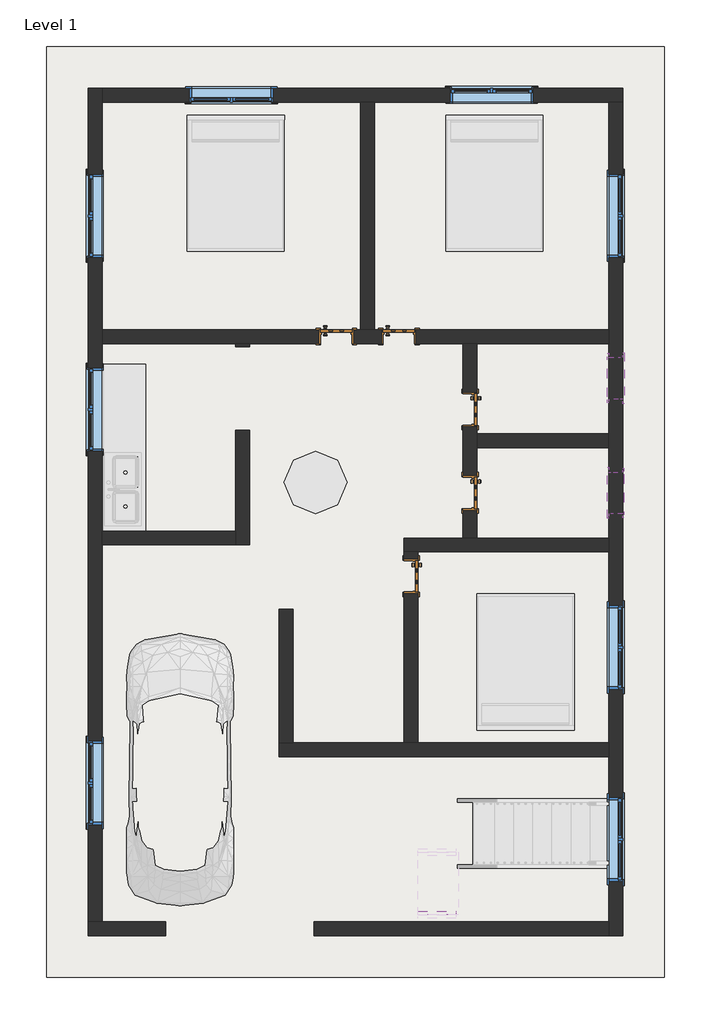
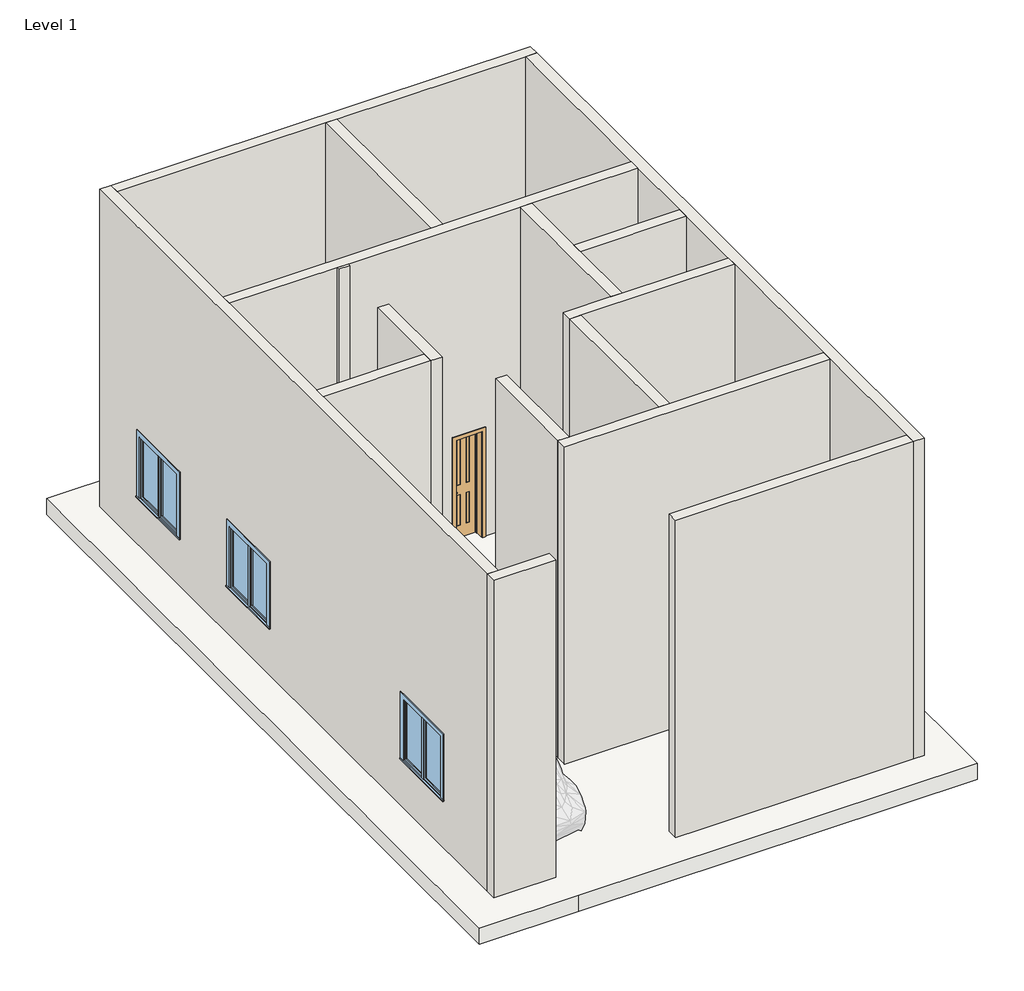
# One storey, part 1 of 2: 16 walls, 10 windows, 5 doors, 1 railing, 1 slab.
"""IFC4 building model written with IfcOpenShell, lengths in millimetres."""

from ifc_helpers import new_model, si_unit, frame, origin, origin_with_axes, place, context, project, spatial, polyline, outline, extrude, faceted_brep, transform, mapped, element, save
from components import door_14995b39, window_0862ab64, window_e41d21a6

model = new_model("IFC4")

# Units and contexts
model_context = context("Model", 3, world=origin())
ifc_project = project(units=[si_unit("LENGTHUNIT", "METRE", prefix="MILLI")], contexts=[model_context])

# Site, building, storey
site = spatial("IfcSite", under=ifc_project)
building = spatial("IfcBuilding", under=site)
storey = spatial("IfcBuildingStorey", under=building, Name="Level 1", Elevation=0.0)

# Doors
placement = place(None, origin())
door_shape = door_14995b39(model_context)
element("IfcDoor", 1, ObjectType="Door-Interior-Single-4_Panel-Wood : 18\" x 80\"", at=placement, inside=storey, context=model_context, shape_type="MappedRepresentation", body=[
    mapped(door_shape, transform((-11008.6836698, 6854.6656775, 0.0), x_axis=(1.0, 0.0, 0.0), y_axis=(0.0, 1.0, 0.0), z_axis=(0.0, 0.0, 1.0))),
])
element("IfcDoor", 2, ObjectType="Door-Interior-Single-4_Panel-Wood : 18\" x 80\"", at=placement, inside=storey, context=model_context, shape_type="MappedRepresentation", body=[
    mapped(door_shape, transform((-10094.2836698, 6854.6656775, 0.0), x_axis=(1.0, 0.0, 0.0), y_axis=(0.0, 1.0, 0.0), z_axis=(0.0, 0.0, 1.0))),
])
element("IfcDoor", 3, ObjectType="Door-Interior-Single-4_Panel-Wood : 18\" x 80\"", at=placement, inside=storey, context=model_context, shape_type="MappedRepresentation", body=[
    mapped(door_shape, transform((-9049.7086698, 5784.6906775, 0.0), x_axis=(0.0, -1.0, 0.0), y_axis=(1.0, 0.0, 0.0), z_axis=(0.0, 0.0, 1.0))),
])
element("IfcDoor", 4, ObjectType="Door-Interior-Single-4_Panel-Wood : 18\" x 80\"", at=placement, inside=storey, context=model_context, shape_type="MappedRepresentation", body=[
    mapped(door_shape, transform((-9049.7086698, 4565.4906775, 0.0), x_axis=(0.0, -1.0, 0.0), y_axis=(1.0, 0.0, 0.0), z_axis=(0.0, 0.0, 1.0))),
])
element("IfcDoor", 5, ObjectType="Door-Interior-Single-4_Panel-Wood : 18\" x 80\"", at=placement, inside=storey, context=model_context, shape_type="MappedRepresentation", body=[
    mapped(door_shape, transform((-9913.3086698, 3346.2906775, 0.0), x_axis=(0.0, -1.0, 0.0), y_axis=(1.0, 0.0, 0.0), z_axis=(0.0, 0.0, 1.0))),
])

# Railing
element("IfcRailing", 6, ObjectType="Handrail - Rectangular", at=placement, inside=storey, context=model_context, shape_type="SweptSolid", body=[
    extrude(outline(polyline([(3115.7333333, -9814.8836698), (3056.3318731, -9814.8836698), (3394.9985397, -9256.0836698), (3454.4, -9256.0836698), (3115.7333333, -9814.8836698)])), frame((0.0, -1606.7093225, 0.0), z_axis=(0.0, 1.0, 0.0), x_axis=(0.0, 0.0, 1.0)), (0.0, 0.0, 1.0), 50.8),
    extrude(outline(polyline([(3081.3470246, -9773.6086698), (2201.3333333, -9773.6086698), (2201.3333333, -9754.5586698), (3092.8924791, -9754.5586698), (3081.3470246, -9773.6086698)])), frame((0.0, -1590.8343225, 0.0), z_axis=(0.0, 1.0, 0.0), x_axis=(0.0, 0.0, 1.0)), (0.0, 0.0, 1.0), 19.05),
    extrude(outline(polyline([(3142.9227822, -9672.0086698), (2201.3333333, -9672.0086698), (2201.3333333, -9652.9586698), (3154.4682367, -9652.9586698), (3142.9227822, -9672.0086698)])), frame((0.0, -1590.8343225, 0.0), z_axis=(0.0, 1.0, 0.0), x_axis=(0.0, 0.0, 1.0)), (0.0, 0.0, 1.0), 19.05),
    extrude(outline(polyline([(3204.4985397, -9570.4086698), (2201.3333333, -9570.4086698), (2201.3333333, -9551.3586698), (3216.0439943, -9551.3586698), (3204.4985397, -9570.4086698)])), frame((0.0, -1590.8343225, 0.0), z_axis=(0.0, 1.0, 0.0), x_axis=(0.0, 0.0, 1.0)), (0.0, 0.0, 1.0), 19.05),
    extrude(outline(polyline([(3266.0742973, -9468.8086698), (2370.6666667, -9468.8086698), (2370.6666667, -9449.7586698), (3277.6197519, -9449.7586698), (3266.0742973, -9468.8086698)])), frame((0.0, -1590.8343225, 0.0), z_axis=(0.0, 1.0, 0.0), x_axis=(0.0, 0.0, 1.0)), (0.0, 0.0, 1.0), 19.05),
    extrude(outline(polyline([(3327.6500549, -9367.2086698), (2370.6666667, -9367.2086698), (2370.6666667, -9348.1586698), (3339.1955094, -9348.1586698), (3327.6500549, -9367.2086698)])), frame((0.0, -1590.8343225, 0.0), z_axis=(0.0, 1.0, 0.0), x_axis=(0.0, 0.0, 1.0)), (0.0, 0.0, 1.0), 19.05),
    extrude(outline(polyline([(3056.3318731, -9814.8836698), (2201.3333333, -9814.8836698), (2201.3333333, -9795.8336698), (3067.8773276, -9795.8336698), (3056.3318731, -9814.8836698)])), frame((0.0, -1590.8343225, 0.0), z_axis=(0.0, 1.0, 0.0), x_axis=(0.0, 0.0, 1.0)), (0.0, 0.0, 1.0), 19.05),
    extrude(outline(polyline([(3383.4530852, -9275.1336698), (2370.6666667, -9275.1336698), (2370.6666667, -9256.0836698), (3394.9985397, -9256.0836698), (3383.4530852, -9275.1336698)])), frame((0.0, -1590.8343225, 0.0), z_axis=(0.0, 1.0, 0.0), x_axis=(0.0, 0.0, 1.0)), (0.0, 0.0, 1.0), 19.05),
])

# Slab
element("IfcSlab", 7, ObjectType="Generic - 12\"", at=placement, inside=storey, context=model_context, shape_type="SweptSolid", body=[
    extrude(outline(polyline([(-15250.4836698, 11093.2906775), (-6208.0836698, 11093.2906775), (-6208.0836698, -2521.1093225), (-13444.0675444, -2521.1093225), (-15250.4836698, -2521.1093225), (-15250.4836698, 11093.2906775)])), frame((0.0, 0.0, -304.8), z_axis=(0.0, 0.0, 1.0), x_axis=(1.0, 0.0, 0.0)), (0.0, 0.0, 1.0), 304.8),
])

# Walls
element("IfcWall", 8, ObjectType="Generic - 8\"", at=placement, inside=storey, context=model_context, shape_type="Brep", body=[
    faceted_brep([(-14437.6836698, 10280.4906775, 0.0), (-10653.0836698, 10280.4906775, 0.0), (-10449.8836698, 10280.4906775, 0.0), (-7020.8836698, 10280.4906775, 0.0), (-6817.6836698, 10280.4906775, 0.0), (-6817.6836698, 10280.4906775, 6096.0), (-7020.8836698, 10280.4906775, 6096.0), (-10449.8836698, 10280.4906775, 6096.0), (-10653.0836698, 10280.4906775, 6096.0), (-14437.6836698, 10280.4906775, 6096.0), (-13154.9836698, 10280.4906775, 2133.6), (-11935.7836698, 10280.4906775, 2133.6), (-11935.7836698, 10280.4906775, 914.4), (-13154.9836698, 10280.4906775, 914.4), (-8125.7836698, 10280.4906775, 2133.6), (-8125.7836698, 10280.4906775, 914.4), (-9344.9836698, 10280.4906775, 914.4), (-9344.9836698, 10280.4906775, 2133.6), (-14437.6836698, 10483.6906775, 0.0), (-14437.6836698, 10483.6906775, 6096.0), (-6817.6836698, 10483.6906775, 6096.0), (-6817.6836698, 10483.6906775, 0.0), (-13154.9836698, 10483.6906775, 2133.6), (-13154.9836698, 10483.6906775, 914.4), (-11935.7836698, 10483.6906775, 914.4), (-11935.7836698, 10483.6906775, 2133.6), (-8125.7836698, 10483.6906775, 2133.6), (-9344.9836698, 10483.6906775, 2133.6), (-9344.9836698, 10483.6906775, 914.4), (-8125.7836698, 10483.6906775, 914.4)], [[[0, 1, 2, 3, 4, 5, 6, 7, 8, 9], [10, 11, 12, 13], [14, 15, 16, 17]], [[18, 19, 20, 21], [22, 23, 24, 25], [26, 27, 28, 29]], [[4, 3, 2, 1, 0, 18, 21]], [[9, 8, 7, 6, 5, 20, 19]], [[5, 4, 21, 20]], [[0, 9, 19, 18]], [[23, 22, 10, 13]], [[24, 23, 13, 12]], [[25, 24, 12, 11]], [[22, 25, 11, 10]], [[15, 14, 26, 29]], [[16, 15, 29, 28]], [[17, 16, 28, 27]], [[14, 17, 27, 26]]]),
])
element("IfcWall", 9, ObjectType="Generic - 8\"", at=placement, inside=storey, context=model_context, shape_type="Brep", body=[
    faceted_brep([(-7020.8836698, 10280.4906775, 0.0), (-7020.8836698, 6953.0906775, 0.0), (-7020.8836698, 6749.8906775, 0.0), (-7020.8836698, 5429.0906775, 0.0), (-7020.8836698, 5225.8906775, 0.0), (-7020.8836698, 3905.0906775, 0.0), (-7020.8836698, 3701.8906775, 0.0), (-7020.8836698, 907.8906775, 0.0), (-7020.8836698, 704.6906775, 0.0), (-7020.8836698, -1708.3093225, 0.0), (-7020.8836698, -1911.5093225, 0.0), (-7020.8836698, -1911.5093225, 6096.0), (-7020.8836698, -1708.3093225, 6096.0), (-7020.8836698, 704.6906775, 6096.0), (-7020.8836698, 907.8906775, 6096.0), (-7020.8836698, 3701.8906775, 6096.0), (-7020.8836698, 3905.0906775, 6096.0), (-7020.8836698, 5225.8906775, 6096.0), (-7020.8836698, 5429.0906775, 6096.0), (-7020.8836698, 6749.8906775, 6096.0), (-7020.8836698, 6953.0906775, 6096.0), (-7020.8836698, 10280.4906775, 6096.0), (-7020.8836698, 8007.1906775, 2133.6), (-7020.8836698, 8007.1906775, 914.4), (-7020.8836698, 9226.3906775, 914.4), (-7020.8836698, 9226.3906775, 2133.6), (-7020.8836698, 1695.2906775, 2133.6), (-7020.8836698, 1695.2906775, 914.4), (-7020.8836698, 2914.4906775, 914.4), (-7020.8836698, 2914.4906775, 2133.6), (-7020.8836698, -1111.4093225, 2133.6), (-7020.8836698, -1111.4093225, 914.4), (-7020.8836698, 107.7906775, 914.4), (-7020.8836698, 107.7906775, 2133.6), (-7020.8836698, 4870.2906775, 2768.6), (-7020.8836698, 4260.6906775, 2768.6), (-7020.8836698, 4260.6906775, 2159.0), (-7020.8836698, 4870.2906775, 2159.0), (-7020.8836698, 5937.0906775, 2768.6), (-7020.8836698, 5937.0906775, 2159.0), (-7020.8836698, 6546.6906775, 2159.0), (-7020.8836698, 6546.6906775, 2768.6), (-6817.6836698, 10280.4906775, 0.0), (-6817.6836698, 10280.4906775, 6096.0), (-6817.6836698, -1911.5093225, 6096.0), (-6817.6836698, -1911.5093225, 0.0), (-6817.6836698, 8007.1906775, 2133.6), (-6817.6836698, 9226.3906775, 2133.6), (-6817.6836698, 9226.3906775, 914.4), (-6817.6836698, 8007.1906775, 914.4), (-6817.6836698, 1695.2906775, 2133.6), (-6817.6836698, 2914.4906775, 2133.6), (-6817.6836698, 2914.4906775, 914.4), (-6817.6836698, 1695.2906775, 914.4), (-6817.6836698, -1111.4093225, 2133.6), (-6817.6836698, 107.7906775, 2133.6), (-6817.6836698, 107.7906775, 914.4), (-6817.6836698, -1111.4093225, 914.4), (-6817.6836698, 4870.2906775, 2768.6), (-6817.6836698, 4870.2906775, 2159.0), (-6817.6836698, 4260.6906775, 2159.0), (-6817.6836698, 4260.6906775, 2768.6), (-6817.6836698, 5937.0906775, 2768.6), (-6817.6836698, 6546.6906775, 2768.6), (-6817.6836698, 6546.6906775, 2159.0), (-6817.6836698, 5937.0906775, 2159.0)], [[[0, 1, 2, 3, 4, 5, 6, 7, 8, 9, 10, 11, 12, 13, 14, 15, 16, 17, 18, 19, 20, 21], [22, 23, 24, 25], [26, 27, 28, 29], [30, 31, 32, 33], [34, 35, 36, 37], [38, 39, 40, 41]], [[42, 43, 44, 45], [46, 47, 48, 49], [50, 51, 52, 53], [54, 55, 56, 57], [58, 59, 60, 61], [62, 63, 64, 65]], [[10, 9, 8, 7, 6, 5, 4, 3, 2, 1, 0, 42, 45]], [[21, 20, 19, 18, 17, 16, 15, 14, 13, 12, 11, 44, 43]], [[0, 21, 43, 42]], [[11, 10, 45, 44]], [[23, 22, 46, 49]], [[24, 23, 49, 48]], [[25, 24, 48, 47]], [[22, 25, 47, 46]], [[27, 26, 50, 53]], [[28, 27, 53, 52]], [[29, 28, 52, 51]], [[26, 29, 51, 50]], [[31, 30, 54, 57]], [[32, 31, 57, 56]], [[33, 32, 56, 55]], [[30, 33, 55, 54]], [[59, 58, 34, 37]], [[60, 59, 37, 36]], [[61, 60, 36, 35]], [[58, 61, 35, 34]], [[39, 38, 62, 65]], [[40, 39, 65, 64]], [[41, 40, 64, 63]], [[38, 41, 63, 62]]]),
])
element("IfcWall", 10, ObjectType="Generic - 8\"", at=placement, inside=storey, context=model_context, shape_type="SweptSolid", body=[
    extrude(outline(polyline([(-11338.8836698, -1708.3093225), (-7020.8836698, -1708.3093225), (-7020.8836698, -1911.5093225), (-11338.8836698, -1911.5093225), (-11338.8836698, -1708.3093225)])), origin_with_axes(), (0.0, 0.0, 1.0), 6096.0),
])
element("IfcWall", 11, ObjectType="Generic - 8\"", at=placement, inside=storey, context=model_context, shape_type="Brep", body=[
    faceted_brep([(-14437.6836698, -1708.3093225, 0.0), (-14437.6836698, 3803.4906775, 0.0), (-14437.6836698, 4006.6906775, 0.0), (-14437.6836698, 6749.8906775, 0.0), (-14437.6836698, 6953.0906775, 0.0), (-14437.6836698, 10280.4906775, 0.0), (-14437.6836698, 10483.6906775, 0.0), (-14437.6836698, 10483.6906775, 6096.0), (-14437.6836698, 10280.4906775, 6096.0), (-14437.6836698, 6953.0906775, 6096.0), (-14437.6836698, 6749.8906775, 6096.0), (-14437.6836698, 4006.6906775, 6096.0), (-14437.6836698, 3803.4906775, 6096.0), (-14437.6836698, -1708.3093225, 6096.0), (-14437.6836698, 9226.3906775, 2133.6), (-14437.6836698, 9226.3906775, 914.4), (-14437.6836698, 8007.1906775, 914.4), (-14437.6836698, 8007.1906775, 2133.6), (-14437.6836698, 6394.2906775, 2133.6), (-14437.6836698, 6394.2906775, 914.4), (-14437.6836698, 5175.0906775, 914.4), (-14437.6836698, 5175.0906775, 2133.6), (-14437.6836698, 933.2906775, 2133.6), (-14437.6836698, 933.2906775, 914.4), (-14437.6836698, -285.9093225, 914.4), (-14437.6836698, -285.9093225, 2133.6), (-14640.8836698, -1708.3093225, 0.0), (-14640.8836698, -1708.3093225, 6096.0), (-14640.8836698, 10483.6906775, 6096.0), (-14640.8836698, 10483.6906775, 0.0), (-14640.8836698, 9226.3906775, 2133.6), (-14640.8836698, 8007.1906775, 2133.6), (-14640.8836698, 8007.1906775, 914.4), (-14640.8836698, 9226.3906775, 914.4), (-14640.8836698, 6394.2906775, 2133.6), (-14640.8836698, 5175.0906775, 2133.6), (-14640.8836698, 5175.0906775, 914.4), (-14640.8836698, 6394.2906775, 914.4), (-14640.8836698, 933.2906775, 2133.6), (-14640.8836698, -285.9093225, 2133.6), (-14640.8836698, -285.9093225, 914.4), (-14640.8836698, 933.2906775, 914.4)], [[[0, 1, 2, 3, 4, 5, 6, 7, 8, 9, 10, 11, 12, 13], [14, 15, 16, 17], [18, 19, 20, 21], [22, 23, 24, 25]], [[26, 27, 28, 29], [30, 31, 32, 33], [34, 35, 36, 37], [38, 39, 40, 41]], [[6, 5, 4, 3, 2, 1, 0, 26, 29]], [[13, 12, 11, 10, 9, 8, 7, 28, 27]], [[0, 13, 27, 26]], [[7, 6, 29, 28]], [[15, 14, 30, 33]], [[16, 15, 33, 32]], [[17, 16, 32, 31]], [[14, 17, 31, 30]], [[19, 18, 34, 37]], [[20, 19, 37, 36]], [[21, 20, 36, 35]], [[18, 21, 35, 34]], [[23, 22, 38, 41]], [[24, 23, 41, 40]], [[25, 24, 40, 39]], [[22, 25, 39, 38]]]),
])
element("IfcWall", 12, ObjectType="Generic - 8\"", at=placement, inside=storey, context=model_context, shape_type="Brep", body=[
    faceted_brep([(-7020.8836698, 6749.8906775, 6096.0), (-8951.2836698, 6749.8906775, 6096.0), (-9154.4836698, 6749.8906775, 6096.0), (-12278.6836698, 6749.8906775, 6096.0), (-12481.8836698, 6749.8906775, 6096.0), (-14437.6836698, 6749.8906775, 6096.0), (-14437.6836698, 6749.8906775, 0.0), (-12481.8836698, 6749.8906775, 0.0), (-12278.6836698, 6749.8906775, 0.0), (-11262.6836698, 6749.8906775, 0.0), (-11262.6836698, 6749.8906775, 2057.4), (-10754.6836698, 6749.8906775, 2057.4), (-10754.6836698, 6749.8906775, 0.0), (-10348.2836698, 6749.8906775, 0.0), (-10348.2836698, 6749.8906775, 2057.4), (-9840.2836698, 6749.8906775, 2057.4), (-9840.2836698, 6749.8906775, 0.0), (-9154.4836698, 6749.8906775, 0.0), (-8951.2836698, 6749.8906775, 0.0), (-7020.8836698, 6749.8906775, 0.0), (-14437.6836698, 6953.0906775, 6096.0), (-10653.0836698, 6953.0906775, 6096.0), (-10449.8836698, 6953.0906775, 6096.0), (-7020.8836698, 6953.0906775, 6096.0), (-7020.8836698, 6953.0906775, 0.0), (-9840.2836698, 6953.0906775, 0.0), (-9840.2836698, 6953.0906775, 2057.4), (-10348.2836698, 6953.0906775, 2057.4), (-10348.2836698, 6953.0906775, 0.0), (-10449.8836698, 6953.0906775, 0.0), (-10653.0836698, 6953.0906775, 0.0), (-10754.6836698, 6953.0906775, 0.0), (-10754.6836698, 6953.0906775, 2057.4), (-11262.6836698, 6953.0906775, 2057.4), (-11262.6836698, 6953.0906775, 0.0), (-14437.6836698, 6953.0906775, 0.0)], [[[0, 1, 2, 3, 4, 5, 6, 7, 8, 9, 10, 11, 12, 13, 14, 15, 16, 17, 18, 19]], [[20, 21, 22, 23, 24, 25, 26, 27, 28, 29, 30, 31, 32, 33, 34, 35]], [[6, 35, 34, 9, 8, 7]], [[24, 19, 18, 17, 16, 25]], [[12, 31, 30, 29, 28, 13]], [[5, 4, 3, 2, 1, 0, 23, 22, 21, 20]], [[0, 19, 24, 23]], [[6, 5, 20, 35]], [[11, 32, 31, 12]], [[32, 11, 10, 33]], [[33, 10, 9, 34]], [[15, 26, 25, 16]], [[26, 15, 14, 27]], [[27, 14, 13, 28]]]),
])
element("IfcWall", 13, ObjectType="Generic - 8\"", at=placement, inside=storey, context=model_context, shape_type="SweptSolid", body=[
    extrude(outline(polyline([(-10449.8836698, 10280.4906775), (-10449.8836698, 6953.0906775), (-10653.0836698, 6953.0906775), (-10653.0836698, 10280.4906775), (-10449.8836698, 10280.4906775)])), origin_with_axes(), (0.0, 0.0, 1.0), 6096.0),
])
element("IfcWall", 14, ObjectType="Generic - 8\"", at=placement, inside=storey, context=model_context, shape_type="SweptSolid", body=[
    extrude(outline(polyline([(-12481.8836698, 3803.4906775), (-14437.6836698, 3803.4906775), (-14437.6836698, 4006.6906775), (-12481.8836698, 4006.6906775), (-12481.8836698, 3803.4906775)])), origin_with_axes(), (0.0, 0.0, 1.0), 6096.0),
])
element("IfcWall", 15, ObjectType="Generic - 8\"", at=placement, inside=storey, context=model_context, shape_type="Brep", body=[
    faceted_brep([(-12278.6836698, 3803.4906775, 0.0), (-12278.6836698, 5479.8906775, 0.0), (-12278.6836698, 5479.8906775, 6096.0), (-12278.6836698, 3803.4906775, 6096.0), (-12481.8836698, 3803.4906775, 0.0), (-12481.8836698, 3803.4906775, 6096.0), (-12481.8836698, 4006.6906775, 6096.0), (-12481.8836698, 5479.8906775, 6096.0), (-12481.8836698, 5479.8906775, 0.0), (-12481.8836698, 4006.6906775, 0.0)], [[[0, 1, 2, 3]], [[4, 5, 6, 7, 8, 9]], [[1, 0, 4, 9, 8]], [[2, 1, 8, 7]], [[3, 2, 7, 6, 5]], [[0, 3, 5, 4]]]),
])
element("IfcWall", 16, ObjectType="Generic - 8\"", at=placement, inside=storey, context=model_context, shape_type="SweptSolid", body=[
    extrude(outline(polyline([(-7020.8836698, 5225.8906775), (-8951.2836698, 5225.8906775), (-8951.2836698, 5429.0906775), (-7020.8836698, 5429.0906775), (-7020.8836698, 5225.8906775)])), origin_with_axes(), (0.0, 0.0, 1.0), 6096.0),
])
element("IfcWall", 17, ObjectType="Generic - 8\"", at=placement, inside=storey, context=model_context, shape_type="Brep", body=[
    faceted_brep([(-10018.0836698, 3701.8906775, 0.0), (-9814.8836698, 3701.8906775, 0.0), (-7020.8836698, 3701.8906775, 0.0), (-7020.8836698, 3701.8906775, 6096.0), (-9814.8836698, 3701.8906775, 6096.0), (-10018.0836698, 3701.8906775, 6096.0), (-10018.0836698, 3905.0906775, 0.0), (-10018.0836698, 3905.0906775, 6096.0), (-9154.4836698, 3905.0906775, 6096.0), (-8951.2836698, 3905.0906775, 6096.0), (-7020.8836698, 3905.0906775, 6096.0), (-7020.8836698, 3905.0906775, 0.0), (-8951.2836698, 3905.0906775, 0.0), (-9154.4836698, 3905.0906775, 0.0)], [[[0, 1, 2, 3, 4, 5]], [[6, 7, 8, 9, 10, 11, 12, 13]], [[2, 1, 0, 6, 13, 12, 11]], [[5, 4, 3, 10, 9, 8, 7]], [[3, 2, 11, 10]], [[0, 5, 7, 6]]]),
])
element("IfcWall", 18, ObjectType="Generic - 8\"", at=placement, inside=storey, context=model_context, shape_type="Brep", body=[
    faceted_brep([(-9154.4836698, 3905.0906775, 6096.0), (-9154.4836698, 6749.8906775, 6096.0), (-9154.4836698, 6749.8906775, 0.0), (-9154.4836698, 6038.6906775, 0.0), (-9154.4836698, 6038.6906775, 2057.4), (-9154.4836698, 5530.6906775, 2057.4), (-9154.4836698, 5530.6906775, 0.0), (-9154.4836698, 4819.4906775, 0.0), (-9154.4836698, 4819.4906775, 2057.4), (-9154.4836698, 4311.4906775, 2057.4), (-9154.4836698, 4311.4906775, 0.0), (-9154.4836698, 3905.0906775, 0.0), (-8951.2836698, 6749.8906775, 6096.0), (-8951.2836698, 5429.0906775, 6096.0), (-8951.2836698, 5225.8906775, 6096.0), (-8951.2836698, 3905.0906775, 6096.0), (-8951.2836698, 3905.0906775, 0.0), (-8951.2836698, 4311.4906775, 0.0), (-8951.2836698, 4311.4906775, 2057.4), (-8951.2836698, 4819.4906775, 2057.4), (-8951.2836698, 4819.4906775, 0.0), (-8951.2836698, 5225.8906775, 0.0), (-8951.2836698, 5429.0906775, 0.0), (-8951.2836698, 5530.6906775, 0.0), (-8951.2836698, 5530.6906775, 2057.4), (-8951.2836698, 6038.6906775, 2057.4), (-8951.2836698, 6038.6906775, 0.0), (-8951.2836698, 6749.8906775, 0.0)], [[[0, 1, 2, 3, 4, 5, 6, 7, 8, 9, 10, 11]], [[12, 13, 14, 15, 16, 17, 18, 19, 20, 21, 22, 23, 24, 25, 26, 27]], [[2, 27, 26, 3]], [[16, 11, 10, 17]], [[6, 23, 22, 21, 20, 7]], [[1, 0, 15, 14, 13, 12]], [[2, 1, 12, 27]], [[0, 11, 16, 15]], [[5, 24, 23, 6]], [[24, 5, 4, 25]], [[25, 4, 3, 26]], [[9, 18, 17, 10]], [[18, 9, 8, 19]], [[19, 8, 7, 20]]]),
])
element("IfcWall", 19, ObjectType="Generic - 8\"", at=placement, inside=storey, context=model_context, shape_type="SweptSolid", body=[
    extrude(outline(polyline([(907.8906775, 6096.0), (3701.8906775, 6096.0), (3701.8906775, 0.0), (3600.2906775, 0.0), (3600.2906775, 2057.4), (3092.2906775, 2057.4), (3092.2906775, 0.0), (907.8906775, 0.0), (907.8906775, 6096.0)])), frame((-10018.0836698, 0.0, 0.0), z_axis=(1.0, 0.0, 0.0), x_axis=(0.0, 1.0, 0.0)), (0.0, 0.0, 1.0), 203.2),
])
element("IfcWall", 20, ObjectType="Generic - 8\"", at=placement, inside=storey, context=model_context, shape_type="Brep", body=[
    faceted_brep([(-11846.8836698, 704.6906775, 0.0), (-7020.8836698, 704.6906775, 0.0), (-7020.8836698, 704.6906775, 6096.0), (-11846.8836698, 704.6906775, 6096.0), (-11846.8836698, 907.8906775, 0.0), (-11846.8836698, 907.8906775, 6096.0), (-11643.6836698, 907.8906775, 6096.0), (-10018.0836698, 907.8906775, 6096.0), (-9814.8836698, 907.8906775, 6096.0), (-7020.8836698, 907.8906775, 6096.0), (-7020.8836698, 907.8906775, 0.0), (-9814.8836698, 907.8906775, 0.0), (-10018.0836698, 907.8906775, 0.0), (-11643.6836698, 907.8906775, 0.0)], [[[0, 1, 2, 3]], [[4, 5, 6, 7, 8, 9, 10, 11, 12, 13]], [[1, 0, 4, 13, 12, 11, 10]], [[3, 2, 9, 8, 7, 6, 5]], [[2, 1, 10, 9]], [[0, 3, 5, 4]]]),
])
element("IfcWall", 21, ObjectType="Generic - 8\"", at=placement, inside=storey, context=model_context, shape_type="SweptSolid", body=[
    extrude(outline(polyline([(-11643.6836698, 2863.6906775), (-11643.6836698, 907.8906775), (-11846.8836698, 907.8906775), (-11846.8836698, 2863.6906775), (-11643.6836698, 2863.6906775)])), origin_with_axes(), (0.0, 0.0, 1.0), 6096.0),
])
element("IfcWall", 22, ObjectType="Generic - 8\"", at=placement, inside=storey, context=model_context, shape_type="Brep", body=[
    faceted_brep([(-13510.5836698, -1708.3093225, 0.0), (-14437.6836698, -1708.3093225, 0.0), (-14640.8836698, -1708.3093225, 0.0), (-14640.8836698, -1708.3093225, 6096.0), (-14437.6836698, -1708.3093225, 6096.0), (-13510.5836698, -1708.3093225, 6096.0), (-13510.5836698, -1911.5093225, 0.0), (-13510.5836698, -1911.5093225, 6096.0), (-14640.8836698, -1911.5093225, 6096.0), (-14640.8836698, -1911.5093225, 0.0)], [[[0, 1, 2, 3, 4, 5]], [[6, 7, 8, 9]], [[2, 1, 0, 6, 9]], [[5, 4, 3, 8, 7]], [[0, 5, 7, 6]], [[3, 2, 9, 8]]]),
])
element("IfcWall", 23, ObjectType="Generic - 8\"", at=placement, inside=storey, context=model_context, shape_type="SweptSolid", body=[
    extrude(outline(polyline([(-12278.6836698, 6749.8906775), (-12278.6836698, 6699.0906775), (-12481.8836698, 6699.0906775), (-12481.8836698, 6749.8906775), (-12278.6836698, 6749.8906775)])), origin_with_axes(), (0.0, 0.0, 1.0), 6096.0),
])

# Windows
window_shape = window_0862ab64(model_context)
element("IfcWindow", 24, ObjectType="Casement Dbl with Trim : 48\" x 48\"", at=placement, inside=storey, context=model_context, shape_type="MappedRepresentation", body=[
    mapped(window_shape, transform((-12545.3836698, 10401.1406775, 0.0), x_axis=(-1.0, 0.0, 0.0), y_axis=(0.0, -1.0, 0.0), z_axis=(0.0, 0.0, 1.0))),
])
element("IfcWindow", 25, ObjectType="Casement Dbl with Trim : 48\" x 48\"", at=placement, inside=storey, context=model_context, shape_type="MappedRepresentation", body=[
    mapped(window_shape, transform((-14520.2336698, 8616.7906775, 0.0), x_axis=(0.0, 1.0, 0.0), y_axis=(-1.0, 0.0, 0.0), z_axis=(0.0, 0.0, 1.0))),
])
element("IfcWindow", 26, ObjectType="Casement Dbl with Trim : 48\" x 48\"", at=placement, inside=storey, context=model_context, shape_type="MappedRepresentation", body=[
    mapped(window_shape, transform((-8735.3836698, 10363.0406775, 0.0), x_axis=(1.0, 0.0, 0.0), y_axis=(0.0, 1.0, 0.0), z_axis=(0.0, 0.0, 1.0))),
])
element("IfcWindow", 27, ObjectType="Casement Dbl with Trim : 48\" x 48\"", at=placement, inside=storey, context=model_context, shape_type="MappedRepresentation", body=[
    mapped(window_shape, transform((-6938.3336698, 8616.7906775, 0.0), x_axis=(0.0, -1.0, 0.0), y_axis=(1.0, 0.0, 0.0), z_axis=(0.0, 0.0, 1.0))),
])
element("IfcWindow", 28, ObjectType="Casement Dbl with Trim : 48\" x 48\"", at=placement, inside=storey, context=model_context, shape_type="MappedRepresentation", body=[
    mapped(window_shape, transform((-14520.2336698, 5784.6906775, 0.0), x_axis=(0.0, 1.0, 0.0), y_axis=(-1.0, 0.0, 0.0), z_axis=(0.0, 0.0, 1.0))),
])
element("IfcWindow", 29, ObjectType="Casement Dbl with Trim : 48\" x 48\"", at=placement, inside=storey, context=model_context, shape_type="MappedRepresentation", body=[
    mapped(window_shape, transform((-6938.3336698, 2304.8906775, 0.0), x_axis=(0.0, -1.0, 0.0), y_axis=(1.0, 0.0, 0.0), z_axis=(0.0, 0.0, 1.0))),
])
element("IfcWindow", 30, ObjectType="Casement Dbl with Trim : 48\" x 48\"", at=placement, inside=storey, context=model_context, shape_type="MappedRepresentation", body=[
    mapped(window_shape, transform((-6938.3336698, -501.8093225, 0.0), x_axis=(0.0, -1.0, 0.0), y_axis=(1.0, 0.0, 0.0), z_axis=(0.0, 0.0, 1.0))),
])
element("IfcWindow", 31, ObjectType="Casement Dbl with Trim : 48\" x 48\"", at=placement, inside=storey, context=model_context, shape_type="MappedRepresentation", body=[
    mapped(window_shape, transform((-14520.2336698, 323.6906775, 0.0), x_axis=(0.0, 1.0, 0.0), y_axis=(-1.0, 0.0, 0.0), z_axis=(0.0, 0.0, 1.0))),
])
window_2_shape = window_e41d21a6(model_context)
element("IfcWindow", 32, ObjectType="Transom with Trim : 24\" x 24\"", at=placement, inside=storey, context=model_context, shape_type="MappedRepresentation", body=[
    mapped(window_2_shape, transform((-6919.2836698, 4603.5906775, 0.0), x_axis=(0.0, 1.0, 0.0), y_axis=(-1.0, 0.0, 0.0), z_axis=(0.0, 0.0, 1.0))),
])
element("IfcWindow", 33, ObjectType="Transom with Trim : 24\" x 24\"", at=placement, inside=storey, context=model_context, shape_type="MappedRepresentation", body=[
    mapped(window_2_shape, transform((-6919.2836698, 6203.7906775, 0.0), x_axis=(0.0, -1.0, 0.0), y_axis=(1.0, 0.0, 0.0), z_axis=(0.0, 0.0, 1.0))),
])

save(model, "model.ifc")

# Revit data of these elements
# Type "Door-Interior-Single-4_Panel-Wood : 18\" x 80\""
#   Type Mark = "8"
#   Assembly Code = "C1020300"
#   Analytic Construction = "Wooden"
#   Top Rail = 0' - 4 11/16"
#   Thickness = 0' - 1 3/8"
#   Thermal Resistance (R) = 2.5876 (h·ft²·°F)/BTU
#   Swing Angle [instance default] = 90.00°
#   Stiles = 0' - 4 3/4"
#   Rough Width = 1' - 8"
#   Rough Height = 6' - 9"
#   Mullion = 0' - 4 1/2"
#   Lock Rail = 0' - 7 1/2"
#   Height = 6' - 8"
#   Width = 1' - 6"
#   Heat Transfer Coefficient (U) = 0.3865 BTU/(h·ft²·°F)
#   Bottom Rail = 0' - 9 1/8"
#   Trim Material = Cherry
#   Panel Material = Cherry
#   Frame Material = Cherry
#   Door Handle Material = Aluminum
#   Visual Light Transmittance = 0
#   Solar Heat Gain Coefficient = 0
#   Wall Closure = (empty or 0)
#   Function = (empty or 0)
# Type "Handrail - Rectangular"
#   Assembly Code = "C2010400"
#   built-in parameter 1008612 = 0.0416667 (stored number, unit not read)
#   built-in parameter 1008611 = 0.0416667 (stored number, unit not read)
#   built-in parameter 1008609 = 0.333333 (stored number, unit not read)
#   built-in parameter 1008604 = 0.166667 (stored number, unit not read)
#   built-in parameter 1008603 = 0.166667 (stored number, unit not read)
#   Railing Height = 3' - 0"
#   built-in parameter 1008630 = 2
#   built-in parameter 1008610 = 2
#   built-in parameter 1008618 = Baluster - Square : 3/4"
# Type "Generic - 12\""
#   Assembly Code = "B1010"
#   Function = 0
#   Layers, outside or top first: 1' - 0" no material (function 1)
# Type "Generic - 8\""
#   Assembly Code = "B2010"
#   Layers, outside or top first: 0' - 8" no material (function 1)
# Type "Casement Dbl with Trim : 48\" x 48\""
#   Type Mark = "10"
#   Construction Type Id = "GSP4R"
#   Assembly Code = "B2020100"
#   Analytic Construction = "1/8 in Pilkington single glazing"
#   Visual Light Transmittance = 0.9
#   Solar Heat Gain Coefficient = 0.78
#   Heat Transfer Coefficient (U) = 0.6496 BTU/(h·ft²·°F)
#   Height = 4' - 0"
#   Default Sill Height = 3' - 0"
#   Trim Projection - Ext. = 0' - 0 1/2"
#   Trim Projection - Int. = 0' - 0 3/4"
#   Trim Width - Exterior = 0' - 3 1/2"
#   Trim Width - Interior = 0' - 3 1/2"
#   Width = 4' - 0"
#   Window Inset = 0' - 0 3/4"
#   Define Thermal Properties by = 1
#   Glass Pane Material = Glass
#   Sash Material = Sash
#   Trim Exterior Material = Trim
#   Trim Interior Material = Trim
#   Wall Closure = (empty or 0)
# Type "Transom with Trim : 24\" x 24\""
#   Type Mark = "13"
#   Construction Type Id = "GSP4R"
#   Assembly Code = "B2020100"
#   Analytic Construction = "1/8 in Pilkington single glazing"
#   Visual Light Transmittance = 0.9
#   Solar Heat Gain Coefficient = 0.78
#   Heat Transfer Coefficient (U) = 0.6496 BTU/(h·ft²·°F)
#   Height = 2' - 0"
#   Default Sill Height = 7' - 1"
#   Trim Projection - Ext. = 0' - 0 1/2"
#   Trim Projection - Int. = 0' - 0 3/4"
#   Trim Width - Exterior = 0' - 3 1/2"
#   Trim Width - Interior = 0' - 3 1/2"
#   Width = 2' - 0"
#   Window Inset = 0' - 0 3/4"
#   Define Thermal Properties by = 1
#   Glass Pane Material = Glass
#   Sash Material = Sash
#   Trim Exterior Material = Trim
#   Trim Interior Material = Trim
#   Wall Closure = (empty or 0)
# Elements 1, 2, 3, 4, 5 (IfcDoor, "Door-Interior-Single-4_Panel-Wood : 18\" x 80\"")
#   Swing Angle = 90.00°
#   Phase Created = New Construction
#   Materials on its faces: "Cherry", "Aluminum"
# Element 6 (IfcRailing, "Handrail - Rectangular")
#   Phase Created = New Construction
# Element 7 (IfcSlab, "Generic - 12\"")
#   built-in parameter 1001955 = 1.5708 (stored number, unit not read)
#   Height Offset From Level = 0' - 0"
#   Phase Created = New Construction
#   Materials on its faces: "Default Floor"
# Elements 8, 9, 10, 11, 12, 13, 14, 15, 16, 17, 18, 19, 20, 21, 22, 23 (IfcWall, "Generic - 8\"")
#   Top Offset = 0' - 0"
#   Base Offset = 0' - 0"
#   Unconnected Height = 20' - 0"
#   wall height = 20' - 0"
#   Phase Created = New Construction
#   Base Constraint = Level 1
#   Materials on its faces: "Default Wall"
# Element 24 (IfcWindow, "Casement Dbl with Trim : 48\" x 48\"")
#   Mark = "1"
#   Phase Created = New Construction
#   Materials on its faces: "Sash", "Trim", "Glass"
# Element 25 (IfcWindow, "Casement Dbl with Trim : 48\" x 48\"")
#   Mark = "2"
#   Phase Created = New Construction
#   Materials on its faces: "Sash", "Trim", "Glass"
# Element 26 (IfcWindow, "Casement Dbl with Trim : 48\" x 48\"")
#   Mark = "3"
#   Phase Created = New Construction
#   Materials on its faces: "Sash", "Trim", "Glass"
# Element 27 (IfcWindow, "Casement Dbl with Trim : 48\" x 48\"")
#   Mark = "4"
#   Phase Created = New Construction
#   Materials on its faces: "Sash", "Trim", "Glass"
# Element 28 (IfcWindow, "Casement Dbl with Trim : 48\" x 48\"")
#   Mark = "5"
#   Phase Created = New Construction
#   Materials on its faces: "Sash", "Trim", "Glass"
# Element 29 (IfcWindow, "Casement Dbl with Trim : 48\" x 48\"")
#   Mark = "6"
#   Phase Created = New Construction
#   Materials on its faces: "Sash", "Trim", "Glass"
# Element 30 (IfcWindow, "Casement Dbl with Trim : 48\" x 48\"")
#   Mark = "7"
#   Phase Created = New Construction
#   Materials on its faces: "Sash", "Trim", "Glass"
# Element 31 (IfcWindow, "Casement Dbl with Trim : 48\" x 48\"")
#   Mark = "8"
#   Phase Created = New Construction
#   Materials on its faces: "Sash", "Trim", "Glass"
# Element 32 (IfcWindow, "Transom with Trim : 24\" x 24\"")
#   Mark = "9"
#   Phase Created = New Construction
#   Materials on its faces: "Sash", "Trim", "Glass"
# Element 33 (IfcWindow, "Transom with Trim : 24\" x 24\"")
#   Mark = "10"
#   Phase Created = New Construction
#   Materials on its faces: "Sash", "Trim", "Glass"
# Materials
#   "Cherry": class "Wood", colour RGB 226 177 128, transparency 0, Description = "Prunus Serotina", Cost = 0
#   "Aluminum": class "Metal", colour RGB 247 247 247, transparency 0, Description = "Aluminum 6061", Cost = 0
#   "Glass": class "Glass", colour RGB 0 128 192, transparency 0.75, Description = "Soda Lime Glass", Cost = 0
#   "Sash": class "Wood", colour RGB 224 178 126, transparency 0
#   "Trim": class "Wood", colour RGB 224 178 126, transparency 0
#   "Default Floor": colour RGB 128 128 128, transparency 0
#   "Default Wall": colour RGB 128 128 128, transparency 0
